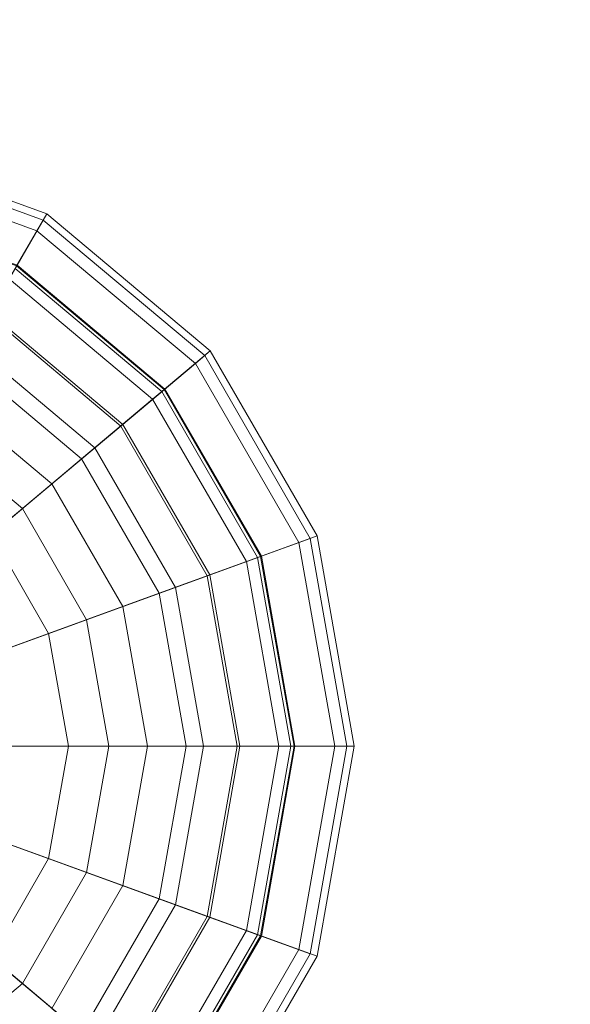
# Model space of a CAD drawing. Units: inches. Extents: x 375 to 1122, y 27 to 1069.
# Tile 111 of 155: x 733.68 to 734.892, y 872.701 to 874.871. Entities that reach past the tile are written whole.
import ezdxf

# ---------------------------------------------------------------- set-up
doc = ezdxf.new("R2010")
doc.units = ezdxf.units.IN
doc.layers.add('A-ANNO-DIMS', color=2, linetype='Continuous', lineweight=18)
doc.layers.add('Furniture', color=30, linetype='Continuous', lineweight=18)
doc.styles.get("Standard").update_dxf_attribs({"font": 'arial.ttf'})
doc.dimstyles.new('ISO-25', dxfattribs={"dimtxt": 12, "dimasz": 2.5, "dimexe": 1.5, "dimexo": 1.5, "dimtad": 1, "dimdec": 1, "dimlunit": 3, "dimtxsty": 'Standard', "dimblk": 'ARCHTICK', "dimcen": 2.5, "dimadec": 0, "dimazin": 0, "dimtfac": 1, "dimtdec": 1, "dimtmove": 0, "dimatfit": 3, "dimfxl": 1.5, "dimfxlon": 1, "dimarcsym": 0})

# ---------------------------------------------------------------- blocks, each defined once
blk = doc.blocks.new('A$C403C54AD')
for points in [[(1.626464, 1.23678, -0.04658), (1.626464, 1.202917, -0.043501), (1.626464, 1.202917, -0.043501), (1.614883, 1.234737, -0.04658)], [(1.626464, 1.233514, -0.043349), (1.626464, 1.23678, -0.04658), (1.614883, 1.234737, -0.04658), (1.616, 1.231669, -0.043349)], [(1.638046, 1.234737, -0.04658), (1.626464, 1.202917, -0.043501), (1.626464, 1.202917, -0.043501), (1.626464, 1.23678, -0.04658)], [(1.636929, 1.231669, -0.043349), (1.638046, 1.234737, -0.04658), (1.626464, 1.23678, -0.04658), (1.626464, 1.233514, -0.043349)], [(1.626464, 1.233473, 0.116404), (1.626464, 1.236381, 0.10318), (1.615019, 1.234363, 0.10318), (1.616013, 1.231631, 0.116404)], [(1.626464, 1.236381, 0.10318), (1.626464, 1.235706, 0.074938), (1.61525, 1.233728, 0.074938), (1.615019, 1.234363, 0.10318)], [(1.636915, 1.231631, 0.116404), (1.637909, 1.234363, 0.10318), (1.626464, 1.236381, 0.10318), (1.626464, 1.233473, 0.116404)], [(1.637909, 1.234363, 0.10318), (1.637678, 1.233728, 0.074938), (1.626464, 1.235706, 0.074938), (1.626464, 1.236381, 0.10318)], [(1.626464, 1.235706, 0.074938), (1.626464, 1.230341, 0.056929), (1.617085, 1.228687, 0.056929), (1.61525, 1.233728, 0.074938)], [(1.637678, 1.233728, 0.074938), (1.635844, 1.228687, 0.056929), (1.626464, 1.230341, 0.056929), (1.626464, 1.235706, 0.074938)], [(1.614883, 1.234737, -0.04658), (1.626464, 1.202917, -0.043501), (1.626464, 1.202917, -0.043501), (1.604698, 1.228857, -0.04658)], [(1.616, 1.231669, -0.043349), (1.614883, 1.234737, -0.04658), (1.604698, 1.228857, -0.04658), (1.606797, 1.226356, -0.043349)], [(1.64823, 1.228857, -0.04658), (1.626464, 1.202917, -0.043501), (1.626464, 1.202917, -0.043501), (1.638046, 1.234737, -0.04658)], [(1.646131, 1.226356, -0.043349), (1.64823, 1.228857, -0.04658), (1.638046, 1.234737, -0.04658), (1.636929, 1.231669, -0.043349)], [(1.616013, 1.231631, 0.116404), (1.615019, 1.234363, 0.10318), (1.604954, 1.228552, 0.10318), (1.606823, 1.226325, 0.116404)], [(1.615019, 1.234363, 0.10318), (1.61525, 1.233728, 0.074938), (1.605388, 1.228035, 0.074938), (1.604954, 1.228552, 0.10318)], [(1.646105, 1.226325, 0.116404), (1.647974, 1.228552, 0.10318), (1.637909, 1.234363, 0.10318), (1.636915, 1.231631, 0.116404)], [(1.647974, 1.228552, 0.10318), (1.64754, 1.228035, 0.074938), (1.637678, 1.233728, 0.074938), (1.637909, 1.234363, 0.10318)], [(1.61525, 1.233728, 0.074938), (1.617085, 1.228687, 0.056929), (1.608836, 1.223925, 0.056929), (1.605388, 1.228035, 0.074938)], [(1.626464, 1.217132, -0.040074), (1.626464, 1.233514, -0.043349), (1.616, 1.231669, -0.043349), (1.621603, 1.216274, -0.040074)], [(1.631326, 1.216274, -0.040074), (1.636929, 1.231669, -0.043349), (1.626464, 1.233514, -0.043349), (1.626464, 1.217132, -0.040074)], [(1.64754, 1.228035, 0.074938), (1.644092, 1.223925, 0.056929), (1.635844, 1.228687, 0.056929), (1.637678, 1.233728, 0.074938)], [(1.626464, 1.228477, 0.12581), (1.626464, 1.233473, 0.116404), (1.616013, 1.231631, 0.116404), (1.617722, 1.226936, 0.12581)], [(1.626464, 1.233296, 0.102963), (1.626464, 1.230487, 0.115599), (1.617035, 1.228824, 0.115599), (1.616074, 1.231464, 0.102963)], [(1.626464, 1.232638, 0.075423), (1.626464, 1.233296, 0.102963), (1.616074, 1.231464, 0.102963), (1.616299, 1.230846, 0.075423)], [(1.635206, 1.226936, 0.12581), (1.636915, 1.231631, 0.116404), (1.626464, 1.233473, 0.116404), (1.626464, 1.228477, 0.12581)], [(1.636854, 1.231464, 0.102963), (1.635893, 1.228824, 0.115599), (1.626464, 1.230487, 0.115599), (1.626464, 1.233296, 0.102963)], [(1.636629, 1.230846, 0.075423), (1.636854, 1.231464, 0.102963), (1.626464, 1.233296, 0.102963), (1.626464, 1.232638, 0.075423)], [(1.626464, 1.227531, 0.058276), (1.626464, 1.232638, 0.075423), (1.616299, 1.230846, 0.075423), (1.618046, 1.226046, 0.058276)], [(1.634882, 1.226046, 0.058276), (1.636629, 1.230846, 0.075423), (1.626464, 1.232638, 0.075423), (1.626464, 1.227531, 0.058276)], [(1.621603, 1.216274, -0.040074), (1.616, 1.231669, -0.043349), (1.606797, 1.226356, -0.043349), (1.617327, 1.213806, -0.040074)], [(1.617722, 1.226936, 0.12581), (1.616013, 1.231631, 0.116404), (1.606823, 1.226325, 0.116404), (1.610035, 1.222497, 0.12581)], [(1.616074, 1.231464, 0.102963), (1.617035, 1.228824, 0.115599), (1.608743, 1.224037, 0.115599), (1.606937, 1.226189, 0.102963)], [(1.616299, 1.230846, 0.075423), (1.616074, 1.231464, 0.102963), (1.606937, 1.226189, 0.102963), (1.60736, 1.225685, 0.075423)], [(1.635601, 1.213806, -0.040074), (1.646131, 1.226356, -0.043349), (1.636929, 1.231669, -0.043349), (1.631326, 1.216274, -0.040074)], [(1.642894, 1.222497, 0.12581), (1.646105, 1.226325, 0.116404), (1.636915, 1.231631, 0.116404), (1.635206, 1.226936, 0.12581)], [(1.645991, 1.226189, 0.102963), (1.644185, 1.224037, 0.115599), (1.635893, 1.228824, 0.115599), (1.636854, 1.231464, 0.102963)], [(1.645568, 1.225685, 0.075423), (1.645991, 1.226189, 0.102963), (1.636854, 1.231464, 0.102963), (1.636629, 1.230846, 0.075423)], [(1.618046, 1.226046, 0.058276), (1.616299, 1.230846, 0.075423), (1.60736, 1.225685, 0.075423), (1.610643, 1.221772, 0.058276)], [(1.642285, 1.221772, 0.058276), (1.645568, 1.225685, 0.075423), (1.636629, 1.230846, 0.075423), (1.634882, 1.226046, 0.058276)], [(1.626464, 1.230487, 0.115599), (1.626464, 1.225399, 0.12581), (1.618775, 1.224043, 0.12581), (1.617035, 1.228824, 0.115599)], [(1.626464, 1.230341, 0.056929), (1.626464, 1.223275, 0.046697), (1.619501, 1.222047, 0.046697), (1.617085, 1.228687, 0.056929)], [(1.635893, 1.228824, 0.115599), (1.634153, 1.224043, 0.12581), (1.626464, 1.225399, 0.12581), (1.626464, 1.230487, 0.115599)], [(1.635844, 1.228687, 0.056929), (1.633427, 1.222047, 0.046697), (1.626464, 1.223275, 0.046697), (1.626464, 1.230341, 0.056929)], [(1.604698, 1.228857, -0.04658), (1.626464, 1.202917, -0.043501), (1.626464, 1.202917, -0.043501), (1.597139, 1.219849, -0.04658)], [(1.606797, 1.226356, -0.043349), (1.604698, 1.228857, -0.04658), (1.597139, 1.219849, -0.04658), (1.599967, 1.218216, -0.043349)], [(1.617035, 1.228824, 0.115599), (1.618775, 1.224043, 0.12581), (1.612014, 1.220139, 0.12581), (1.608743, 1.224037, 0.115599)], [(1.617085, 1.228687, 0.056929), (1.619501, 1.222047, 0.046697), (1.613379, 1.218512, 0.046697), (1.608836, 1.223925, 0.056929)], [(1.65579, 1.219849, -0.04658), (1.626464, 1.202917, -0.043501), (1.626464, 1.202917, -0.043501), (1.64823, 1.228857, -0.04658)], [(1.644092, 1.223925, 0.056929), (1.63955, 1.218512, 0.046697), (1.633427, 1.222047, 0.046697), (1.635844, 1.228687, 0.056929)], [(1.644185, 1.224037, 0.115599), (1.640915, 1.220139, 0.12581), (1.634153, 1.224043, 0.12581), (1.635893, 1.228824, 0.115599)], [(1.606823, 1.226325, 0.116404), (1.604954, 1.228552, 0.10318), (1.597484, 1.219649, 0.10318), (1.600002, 1.218195, 0.116404)], [(1.604954, 1.228552, 0.10318), (1.605388, 1.228035, 0.074938), (1.598069, 1.219312, 0.074938), (1.597484, 1.219649, 0.10318)], [(1.626464, 1.225399, 0.12581), (1.626464, 1.228477, 0.12581), (1.617722, 1.226936, 0.12581), (1.618775, 1.224043, 0.12581)], [(1.634153, 1.224043, 0.12581), (1.635206, 1.226936, 0.12581), (1.626464, 1.228477, 0.12581), (1.626464, 1.225399, 0.12581)], [(1.605388, 1.228035, 0.074938), (1.608836, 1.223925, 0.056929), (1.602714, 1.216629, 0.056929), (1.598069, 1.219312, 0.074938)], [(1.626464, 1.221045, 0.048884), (1.626464, 1.227531, 0.058276), (1.618046, 1.226046, 0.058276), (1.620264, 1.219951, 0.048884)], [(1.632664, 1.219951, 0.048884), (1.634882, 1.226046, 0.058276), (1.626464, 1.227531, 0.058276), (1.626464, 1.221045, 0.048884)], [(1.618775, 1.224043, 0.12581), (1.617722, 1.226936, 0.12581), (1.610035, 1.222497, 0.12581), (1.612014, 1.220139, 0.12581)], [(1.640915, 1.220139, 0.12581), (1.642894, 1.222497, 0.12581), (1.635206, 1.226936, 0.12581), (1.634153, 1.224043, 0.12581)], [(1.617327, 1.213806, -0.040074), (1.606797, 1.226356, -0.043349), (1.599967, 1.218216, -0.043349), (1.614154, 1.210025, -0.040074)], [(1.610035, 1.222497, 0.12581), (1.606823, 1.226325, 0.116404), (1.600002, 1.218195, 0.116404), (1.604329, 1.215697, 0.12581)], [(1.606937, 1.226189, 0.102963), (1.608743, 1.224037, 0.115599), (1.602589, 1.216702, 0.115599), (1.600155, 1.218107, 0.102963)], [(1.60736, 1.225685, 0.075423), (1.606937, 1.226189, 0.102963), (1.600155, 1.218107, 0.102963), (1.600725, 1.217778, 0.075423)], [(1.620264, 1.219951, 0.048884), (1.618046, 1.226046, 0.058276), (1.610643, 1.221772, 0.058276), (1.614812, 1.216804, 0.048884)], [(1.638116, 1.216804, 0.048884), (1.642285, 1.221772, 0.058276), (1.634882, 1.226046, 0.058276), (1.632664, 1.219951, 0.048884)], [(1.638774, 1.210025, -0.040074), (1.652961, 1.218216, -0.043349), (1.646131, 1.226356, -0.043349), (1.635601, 1.213806, -0.040074)], [(1.610643, 1.221772, 0.058276), (1.60736, 1.225685, 0.075423), (1.600725, 1.217778, 0.075423), (1.605149, 1.215224, 0.058276)], [(1.608743, 1.224037, 0.115599), (1.612014, 1.220139, 0.12581), (1.606995, 1.214158, 0.12581), (1.602589, 1.216702, 0.115599)], [(1.608836, 1.223925, 0.056929), (1.613379, 1.218512, 0.046697), (1.608834, 1.213096, 0.046697), (1.602714, 1.216629, 0.056929)], [(1.650214, 1.216629, 0.056929), (1.644094, 1.213096, 0.046697), (1.63955, 1.218512, 0.046697), (1.644092, 1.223925, 0.056929)], [(1.626464, 1.223275, 0.046697), (1.626464, 1.213036, 0.03933), (1.623003, 1.212426, 0.03933), (1.619501, 1.222047, 0.046697)], [(1.633427, 1.222047, 0.046697), (1.629925, 1.212426, 0.03933), (1.626464, 1.213036, 0.03933), (1.626464, 1.223275, 0.046697)], [(1.612014, 1.220139, 0.12581), (1.610035, 1.222497, 0.12581), (1.604329, 1.215697, 0.12581), (1.606995, 1.214158, 0.12581)], [(1.614812, 1.216804, 0.048884), (1.610643, 1.221772, 0.058276), (1.605149, 1.215224, 0.058276), (1.610766, 1.211981, 0.048884)], [(1.619501, 1.222047, 0.046697), (1.623003, 1.212426, 0.03933), (1.61996, 1.210669, 0.03933), (1.613379, 1.218512, 0.046697)], [(1.63955, 1.218512, 0.046697), (1.632968, 1.210669, 0.03933), (1.629925, 1.212426, 0.03933), (1.633427, 1.222047, 0.046697)], [(1.642163, 1.211981, 0.048884), (1.64778, 1.215224, 0.058276), (1.642285, 1.221772, 0.058276), (1.638116, 1.216804, 0.048884)], [(1.626464, 1.211822, 0.042248), (1.626464, 1.221045, 0.048884), (1.620264, 1.219951, 0.048884), (1.623419, 1.211285, 0.042248)], [(1.62951, 1.211285, 0.042248), (1.632664, 1.219951, 0.048884), (1.626464, 1.221045, 0.048884), (1.626464, 1.211822, 0.042248)], [(1.623419, 1.211285, 0.042248), (1.620264, 1.219951, 0.048884), (1.614812, 1.216804, 0.048884), (1.620741, 1.209738, 0.042248)], [(1.632188, 1.209738, 0.042248), (1.638116, 1.216804, 0.048884), (1.632664, 1.219951, 0.048884), (1.62951, 1.211285, 0.042248)], [(1.597139, 1.219849, -0.04658), (1.626464, 1.202917, -0.043501), (1.626464, 1.202917, -0.043501), (1.593116, 1.208798, -0.04658)], [(1.599967, 1.218216, -0.043349), (1.597139, 1.219849, -0.04658), (1.593116, 1.208798, -0.04658), (1.596333, 1.20823, -0.043349)], [(1.600002, 1.218195, 0.116404), (1.597484, 1.219649, 0.10318), (1.593509, 1.208728, 0.10318), (1.596372, 1.208223, 0.116404)], [(1.597484, 1.219649, 0.10318), (1.598069, 1.219312, 0.074938), (1.594174, 1.208611, 0.074938), (1.593509, 1.208728, 0.10318)], [(1.659812, 1.208798, -0.04658), (1.626464, 1.202917, -0.043501), (1.626464, 1.202917, -0.043501), (1.65579, 1.219849, -0.04658)], [(1.598069, 1.219312, 0.074938), (1.602714, 1.216629, 0.056929), (1.599457, 1.20768, 0.056929), (1.594174, 1.208611, 0.074938)], [(1.613379, 1.218512, 0.046697), (1.61996, 1.210669, 0.03933), (1.617701, 1.207977, 0.03933), (1.608834, 1.213096, 0.046697)], [(1.644094, 1.213096, 0.046697), (1.635227, 1.207977, 0.03933), (1.632968, 1.210669, 0.03933), (1.63955, 1.218512, 0.046697)]]:
    blk.add_3dface(points)
blk = doc.blocks.new('_ArchTick')
at = {"color": 0, "linetype": 'ByBlock', "const_width": 0.15}
blk.add_lwpolyline([(-0.5, -0.5), (0.5, 0.5)], dxfattribs=at)
blk = doc.blocks.new('*D88')
at = {"layer": 'A-ANNO-DIMS', "color": 0, "lineweight": -2, "transparency": 16777216}
for p, q in [((731.0073, 1052.5277), (731.0073, 1055.5277)), ((854.0073, 1052.5277), (854.0073, 1055.5277)), ((731.0073, 1054.0277), (854.0073, 1054.0277))]:
    blk.add_line(p, q, dxfattribs=at)
at = {"layer": 'Defpoints', "color": 0, "transparency": 16777216}
for p in [(854.0073, 1054.0277), (731.0073, 502.5277), (854.0073, 502.5277)]:
    blk.add_point(p, dxfattribs=at)
at = {"layer": 'A-ANNO-DIMS', "color": 0, "lineweight": -2, "transparency": 16777216, "xscale": 2.5, "yscale": 2.5, "zscale": 2.5, "rotation": 180}
blk.add_blockref('_ArchTick', (731.0073, 1054.0277), dxfattribs=at)
at = {"layer": 'A-ANNO-DIMS', "color": 0, "lineweight": -2, "transparency": 16777216, "xscale": 2.5, "yscale": 2.5, "zscale": 2.5}
blk.add_blockref('_ArchTick', (854.0073, 1054.0277), dxfattribs=at)
at = {"layer": 'A-ANNO-DIMS', "color": 0, "transparency": 16777216, "insert": (792.5073, 1060.7837), "char_height": 12, "attachment_point": 5}
blk.add_mtext('10\'-3"', dxfattribs=at)
blk = doc.blocks.new('*D91')
at = {"layer": 'A-ANNO-DIMS', "color": 0, "lineweight": -2, "transparency": 16777216}
for p, q in [((728.0073, 1052.5277), (728.0073, 1055.5277)), ((788.0073, 1052.5277), (788.0073, 1055.5277)), ((728.0073, 1054.0277), (788.0073, 1054.0277))]:
    blk.add_line(p, q, dxfattribs=at)
at = {"layer": 'Defpoints', "color": 0, "transparency": 16777216}
for p in [(788.0073, 1054.0277), (728.0073, 774.0277), (788.0073, 774.0277)]:
    blk.add_point(p, dxfattribs=at)
at = {"layer": 'A-ANNO-DIMS', "color": 0, "lineweight": -2, "transparency": 16777216, "xscale": 2.5, "yscale": 2.5, "zscale": 2.5, "rotation": 180}
blk.add_blockref('_ArchTick', (728.0073, 1054.0277), dxfattribs=at)
at = {"layer": 'A-ANNO-DIMS', "color": 0, "lineweight": -2, "transparency": 16777216, "xscale": 2.5, "yscale": 2.5, "zscale": 2.5}
blk.add_blockref('_ArchTick', (788.0073, 1054.0277), dxfattribs=at)
at = {"layer": 'A-ANNO-DIMS', "color": 0, "transparency": 16777216, "insert": (758.0073, 1060.7796), "char_height": 12, "attachment_point": 5}
blk.add_mtext('5\'-0"', dxfattribs=at)

msp = doc.modelspace()

# ---------------------------------------------------------------- block references
at = {"layer": 'Furniture', "xscale": 39.9918517141215, "yscale": 39.9918517141215, "zscale": 39.9918517141215, "rotation": 270}
msp.add_blockref('A$C403C54AD', (684.9549, 938.3156, 0.024), dxfattribs=at)

# ---------------------------------------------------------------- dimensions: what is measured, and where the dimension line sits
at = {"layer": 'A-ANNO-DIMS'}
for base, p1, p2, picture, middle in [((788.0073, 1054.0277), (728.0073, 774.0277), (788.0073, 774.0277), '*D91', (758.0073, 1060.7796)), ((854.0073, 1054.0277), (731.0073, 502.5277), (854.0073, 502.5277), '*D88', (792.5073, 1060.7837))]:
    dim = msp.add_linear_dim(base=base, p1=p1, p2=p2, dimstyle='ISO-25', override={"dimdec": 1, "dimlfac": 1, "dimrnd": 0, "dimzin": 1, "dimdsep": 46, "dimlunit": 4, "dimfrac": 2}, dxfattribs=at)
    dim.commit()
    dim.dimension.update_dxf_attribs({"geometry": picture, "text_midpoint": middle})

doc.saveas('drawing.dxf')
